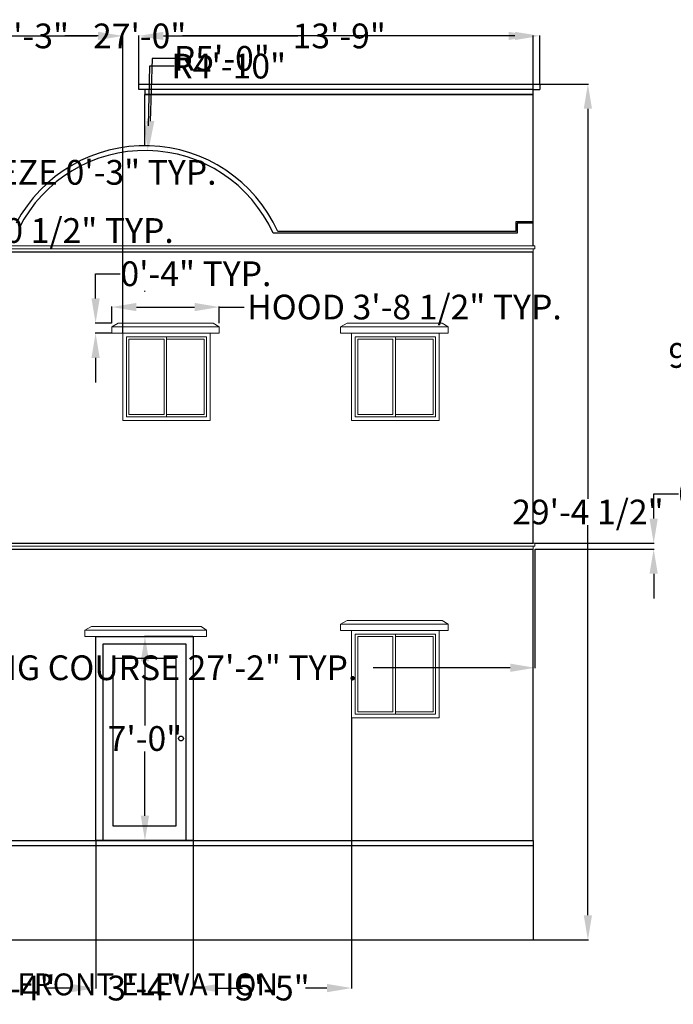
# Model space of a CAD drawing. Units: inches. Extents: x 2393 to 3270, y 740 to 1442.
# Tile 3 of 5: x 2554 to 2823, y 1031 to 1436. Entities that reach past the tile are written whole.
import ezdxf

# ---------------------------------------------------------------- set-up
doc = ezdxf.new("R2010")
doc.units = ezdxf.units.IN
doc.header["$MEASUREMENT"] = 0
for name, color, linetype, lineweight in [('A-ANNO-DIMS', 2, 'Continuous', 18), ('A-ANNO-TITL', 7, 'Continuous', 25), ('A-DOOR', 3, 'Continuous', 25), ('A-ELEV', 7, 'Continuous', 30), ('A-ELEV-TRIM', 8, 'Continuous', 13), ('A-GLAZ', 4, 'Continuous', 18), ('A-ROOF', 7, 'Continuous', 25)]:
    doc.layers.add(name, color=color, linetype=linetype, lineweight=lineweight)
doc.styles.get("Standard").update_dxf_attribs({"font": 'arial.ttf'})
doc.dimstyles.get("Standard").update_dxf_attribs({"dimtxt": 10.18, "dimasz": 10.18, "dimexe": 0.18, "dimexo": 0.0625, "dimgap": 0.09, "dimtad": 0, "dimtih": 1, "dimtoh": 1, "dimdec": 0, "dimzin": 0, "dimdsep": 46, "dimlunit": 3, "dimtxsty": 'Standard', "dimcen": 0.09, "dimadec": 0, "dimazin": 0, "dimtfac": 1, "dimtdec": 0, "dimtofl": 0, "dimtmove": 0, "dimatfit": 3, "dimfxl": 1, "dimtolj": 1, "dimtzin": 0, "dimarcsym": 0})

# ---------------------------------------------------------------- blocks, each defined once
blk = doc.blocks.new('*U7')
blk.add_lwpolyline([(3.12, 0.01), (0.12, 0.01), (0.12, 84.01), (40.12, 84.01), (40.12, 0.01), (37.12, 0.01)])
for points in [[(37.12, 80.99), (37.12, 0.01), (3.12, 0.01), (3.12, 80.99)], [(33.12, 6.01), (33.12, 74.99), (7.12, 74.99), (7.12, 6.01)]]:
    blk.add_lwpolyline(points, close=True)
blk.add_circle((35.12, 42.01), 1)
blk = doc.blocks.new('*U4')
for p, q in [((1.5, 1.5), (1.5, 34.5)), ((1.5, 34.5), (18, 34.5)), ((18, 1.5), (18, 34.5)), ((18, 34.5), (34.5, 34.5)), ((34.5, 34.5), (34.5, 1.5)), ((18, 1.5), (1.5, 1.5)), ((34.5, 1.5), (18, 1.5))]:
    blk.add_line(p, q)
blk.add_lwpolyline([(0, 0), (0, 36), (36, 36), (36, 0)], close=True)
for points in [[(17, 33.5), (17, 2.5), (2.5, 2.5), (2.5, 33.5), (17, 33.5)], [(18, 33.5), (33.5, 33.5), (33.5, 2.5), (18, 2.5)]]:
    blk.add_lwpolyline(points)
blk = doc.blocks.new('WIN-HEAD-HOOD-ELEV')
for p, q in [((0, 2.55), (2.7, 4.11)), ((2.7, 4.11), (41.79, 4.11)), ((41.79, 4.11), (44.29, 2.55)), ((0, 0), (0, 2.55)), ((0, 2.55), (44.29, 2.55)), ((0, 0), (4.55, 0)), ((44.29, 0), (40.55, 0)), ((44.29, 2.55), (44.29, 0))]:
    blk.add_line(p, q)
blk = doc.blocks.new('FACADE-STRING-COURSE')
for p, q in [((0.49, 2.4), (0, 2.4)), ((0, 2.4), (0, 1.23)), ((0, 1.23), (1.17, 1.23)), ((0.49, 2.4), (325.84, 2.4)), ((325.84, 1.23), (325.17, 1.23)), ((325.84, 2.4), (325.84, 1.23))]:
    blk.add_line(p, q)
blk.add_lwpolyline([(1.17, 0), (325.17, 0), (325.17, 1.23), (1.17, 1.23)], close=True)
blk = doc.blocks.new('*D36')
at = {"layer": 'A-ANNO-DIMS', "color": 0, "lineweight": -2, "transparency": 16777216}
for p, q in [((2591.91, 1311.5), (2591.91, 1318.26)), ((2602.09, 1318.08), (2626.02, 1318.08)), ((2636.2, 1311.5), (2636.2, 1318.26)), ((2636.2, 1318.08), (2646.38, 1318.08))]:
    blk.add_line(p, q, dxfattribs=at)
at = {"layer": 'A-ANNO-DIMS', "color": 0, "transparency": 16777216}
for points in [[(2602.09, 1319.77), (2602.09, 1316.38), (2591.91, 1318.08)], [(2626.02, 1319.77), (2626.02, 1316.38), (2636.2, 1318.08)]]:
    blk.add_solid(points, dxfattribs=at)
at = {"layer": 'Defpoints', "color": 0, "transparency": 16777216}
for p in [(2636.2, 1318.08), (2591.91, 1311.43), (2636.2, 1311.43)]:
    blk.add_point(p, dxfattribs=at)
at = {"layer": 'A-ANNO-DIMS', "color": 0, "transparency": 16777216, "insert": (2712.39, 1318.08), "char_height": 10.18, "attachment_point": 5}
blk.add_mtext('\\A1;HOOD 3\'-8 1/2" TYP.', dxfattribs=at)
blk = doc.blocks.new('*D37')
at = {"layer": 'A-ANNO-DIMS', "color": 0, "lineweight": -2, "transparency": 16777216}
for p, q in [((2585.27, 1321.61), (2585.27, 1331.79)), ((2585.27, 1331.79), (2595.45, 1331.79)), ((2591.85, 1311.43), (2585.09, 1311.43)), ((2591.85, 1307.33), (2585.09, 1307.33)), ((2585.27, 1297.15), (2585.27, 1286.97))]:
    blk.add_line(p, q, dxfattribs=at)
at = {"layer": 'A-ANNO-DIMS', "color": 0, "transparency": 16777216}
for points in [[(2583.57, 1321.61), (2586.97, 1321.61), (2585.27, 1311.43)], [(2583.57, 1297.15), (2586.97, 1297.15), (2585.27, 1307.33)]]:
    blk.add_solid(points, dxfattribs=at)
at = {"layer": 'Defpoints', "color": 0, "transparency": 16777216}
for p in [(2585.27, 1311.43), (2591.91, 1311.43), (2591.91, 1307.33)]:
    blk.add_point(p, dxfattribs=at)
at = {"layer": 'A-ANNO-DIMS', "color": 0, "transparency": 16777216, "insert": (2626.57, 1331.79), "char_height": 10.18, "attachment_point": 5}
blk.add_mtext('\\A1;0\'-4" TYP.', dxfattribs=at)
blk = doc.blocks.new('*D38')
at = {"layer": 'A-ANNO-DIMS', "color": 0, "lineweight": -2, "transparency": 16777216}
for p, q in [((2511.53, 1363.37), (2511.53, 1373.55)), ((2511.53, 1373.55), (2521.71, 1373.55)), ((2511.12, 1353.19), (2511.71, 1353.19)), ((2511.12, 1350.06), (2511.71, 1350.06)), ((2511.53, 1339.88), (2511.53, 1329.7))]:
    blk.add_line(p, q, dxfattribs=at)
at = {"layer": 'A-ANNO-DIMS', "color": 0, "transparency": 16777216}
for points in [[(2509.83, 1363.37), (2513.22, 1363.37), (2511.53, 1353.19)], [(2509.83, 1339.88), (2513.22, 1339.88), (2511.53, 1350.06)]]:
    blk.add_solid(points, dxfattribs=at)
at = {"layer": 'Defpoints', "color": 0, "transparency": 16777216}
for p in [(2511.06, 1353.19), (2511.06, 1350.06), (2511.53, 1353.19)]:
    blk.add_point(p, dxfattribs=at)
at = {"layer": 'A-ANNO-DIMS', "color": 0, "transparency": 16777216, "insert": (2579.79, 1373.55), "char_height": 10.18, "attachment_point": 5}
blk.add_mtext('\\A1;FRIEZE 0\'-3" TYP.', dxfattribs=at)
blk = doc.blocks.new('*D39')
at = {"layer": 'A-ANNO-DIMS', "color": 0, "lineweight": -2, "transparency": 16777216}
for p, q in [((2500.38, 1349.6), (2490.2, 1349.6)), ((2510.56, 1350), (2510.56, 1349.42)), ((2511.06, 1350), (2511.06, 1349.42)), ((2521.24, 1349.6), (2531.42, 1349.6))]:
    blk.add_line(p, q, dxfattribs=at)
at = {"layer": 'A-ANNO-DIMS', "color": 0, "transparency": 16777216}
for points in [[(2500.38, 1351.29), (2500.38, 1347.9), (2510.56, 1349.6)], [(2521.24, 1351.29), (2521.24, 1347.9), (2511.06, 1349.6)]]:
    blk.add_solid(points, dxfattribs=at)
at = {"layer": 'Defpoints', "color": 0, "transparency": 16777216}
for p in [(2510.56, 1350.06), (2511.06, 1350.06), (2511.06, 1349.6)]:
    blk.add_point(p, dxfattribs=at)
at = {"layer": 'A-ANNO-DIMS', "color": 0, "transparency": 16777216, "insert": (2574.39, 1349.6), "char_height": 10.18, "attachment_point": 5}
blk.add_mtext('\\A1;0\'-0 1/2" TYP.', dxfattribs=at)
blk = doc.blocks.new('*D40')
at = {"layer": 'A-ANNO-DIMS', "color": 0, "lineweight": -2, "transparency": 16777216}
for p, q in [((2440.26, 1218.37), (2440.26, 1169.38)), ((2766.1, 1218.37), (2766.1, 1169.38)), ((2450.44, 1169.56), (2506.89, 1169.56)), ((2755.92, 1169.56), (2699.46, 1169.56))]:
    blk.add_line(p, q, dxfattribs=at)
at = {"layer": 'A-ANNO-DIMS', "color": 0, "transparency": 16777216}
for points in [[(2450.44, 1171.25), (2450.44, 1167.86), (2440.26, 1169.56)], [(2755.92, 1171.25), (2755.92, 1167.86), (2766.1, 1169.56)]]:
    blk.add_solid(points, dxfattribs=at)
at = {"layer": 'Defpoints', "color": 0, "transparency": 16777216}
for p in [(2440.26, 1218.43), (2766.1, 1218.43), (2766.1, 1169.56)]:
    blk.add_point(p, dxfattribs=at)
at = {"layer": 'A-ANNO-DIMS', "color": 0, "transparency": 16777216, "insert": (2603.18, 1169.56), "char_height": 10.18, "attachment_point": 5}
blk.add_mtext('\\A1;STRING COURSE 27\'-2" TYP.', dxfattribs=at)
blk = doc.blocks.new('*D41')
at = {"layer": 'A-ANNO-DIMS', "color": 0, "lineweight": -2, "transparency": 16777216}
for p, q in [((2814.97, 1231.01), (2814.97, 1241.19)), ((2814.97, 1241.19), (2825.15, 1241.19)), ((2766.16, 1220.83), (2815.15, 1220.83)), ((2766.16, 1218.43), (2815.15, 1218.43)), ((2814.97, 1208.25), (2814.97, 1198.07))]:
    blk.add_line(p, q, dxfattribs=at)
at = {"layer": 'A-ANNO-DIMS', "color": 0, "transparency": 16777216}
for points in [[(2813.27, 1231.01), (2816.67, 1231.01), (2814.97, 1220.83)], [(2813.27, 1208.25), (2816.67, 1208.25), (2814.97, 1218.43)]]:
    blk.add_solid(points, dxfattribs=at)
at = {"layer": 'Defpoints', "color": 0, "transparency": 16777216}
for p in [(2766.1, 1220.83), (2814.97, 1220.83), (2766.1, 1218.43)]:
    blk.add_point(p, dxfattribs=at)
at = {"layer": 'A-ANNO-DIMS', "color": 0, "transparency": 16777216, "insert": (2868.13, 1241.19), "char_height": 10.18, "attachment_point": 5}
blk.add_mtext('\\A1;0\'-2 1/2" TYP.', dxfattribs=at)
blk = doc.blocks.new('*D57')
at = {"layer": 'A-ANNO-DIMS', "color": 0, "lineweight": -2, "transparency": 16777216}
for p, q in [((2441.43, 1353.25), (2441.43, 1429.9)), ((2451.61, 1429.72), (2585.76, 1429.72)), ((2755.25, 1429.72), (2621.09, 1429.72)), ((2765.43, 1353.25), (2765.43, 1429.9))]:
    blk.add_line(p, q, dxfattribs=at)
at = {"layer": 'A-ANNO-DIMS', "color": 0, "transparency": 16777216}
for points in [[(2451.61, 1431.41), (2451.61, 1428.02), (2441.43, 1429.72)], [(2755.25, 1431.41), (2755.25, 1428.02), (2765.43, 1429.72)]]:
    blk.add_solid(points, dxfattribs=at)
at = {"layer": 'Defpoints', "color": 0, "transparency": 16777216}
for p in [(2765.43, 1429.72), (2441.43, 1353.19), (2765.43, 1353.19)]:
    blk.add_point(p, dxfattribs=at)
at = {"layer": 'A-ANNO-DIMS', "color": 0, "transparency": 16777216, "insert": (2603.43, 1429.72), "char_height": 10.18, "attachment_point": 5}
blk.add_mtext('\\A1;27\'-0"', dxfattribs=at)
blk = doc.blocks.new('*D58')
at = {"layer": 'A-ANNO-DIMS', "color": 0, "lineweight": -2, "transparency": 16777216}
for p, q in [((2768.12, 1409.88), (2788.08, 1409.88)), ((2787.9, 1399.7), (2787.9, 1239.05)), ((2787.9, 1067.68), (2787.9, 1228.34)), ((2765.49, 1057.5), (2788.08, 1057.5))]:
    blk.add_line(p, q, dxfattribs=at)
at = {"layer": 'A-ANNO-DIMS', "color": 0, "transparency": 16777216}
for points in [[(2786.2, 1399.7), (2789.59, 1399.7), (2787.9, 1409.88)], [(2786.2, 1067.68), (2789.59, 1067.68), (2787.9, 1057.5)]]:
    blk.add_solid(points, dxfattribs=at)
at = {"layer": 'Defpoints', "color": 0, "transparency": 16777216}
for p in [(2768.06, 1409.88), (2787.9, 1409.88), (2765.43, 1057.5)]:
    blk.add_point(p, dxfattribs=at)
at = {"layer": 'A-ANNO-DIMS', "color": 0, "transparency": 16777216, "insert": (2787.9, 1233.69), "char_height": 10.18, "attachment_point": 5}
blk.add_mtext('\\A1;29\'-4 1/2"', dxfattribs=at)
blk = doc.blocks.new('*D66')
at = {"layer": 'A-ANNO-DIMS', "color": 0, "lineweight": -2, "transparency": 16777216}
for p, q in [((2625.36, 1182.43), (2605.41, 1182.43)), ((2605.59, 1172.25), (2605.59, 1145.72)), ((2605.59, 1108.61), (2605.59, 1135.14)), ((2625.36, 1098.43), (2605.41, 1098.43))]:
    blk.add_line(p, q, dxfattribs=at)
at = {"layer": 'A-ANNO-DIMS', "color": 0, "transparency": 16777216}
for points in [[(2603.89, 1172.25), (2607.29, 1172.25), (2605.59, 1182.43)], [(2603.89, 1108.61), (2607.29, 1108.61), (2605.59, 1098.43)]]:
    blk.add_solid(points, dxfattribs=at)
at = {"layer": 'Defpoints', "color": 0, "transparency": 16777216}
for p in [(2605.59, 1182.43), (2625.43, 1182.43), (2625.43, 1098.43)]:
    blk.add_point(p, dxfattribs=at)
at = {"layer": 'A-ANNO-DIMS', "color": 0, "transparency": 16777216, "insert": (2605.59, 1140.43), "char_height": 10.18, "attachment_point": 5}
blk.add_mtext('\\A1;7\'-0"', dxfattribs=at)
blk = doc.blocks.new('*D69')
at = {"layer": 'A-ANNO-DIMS', "color": 0, "lineweight": -2, "transparency": 16777216}
for p, q in [((2521.51, 1148.87), (2521.51, 1037.49)), ((2585.43, 1098.37), (2585.43, 1037.49)), ((2531.69, 1037.67), (2539.85, 1037.67)), ((2575.25, 1037.67), (2567.09, 1037.67))]:
    blk.add_line(p, q, dxfattribs=at)
at = {"layer": 'A-ANNO-DIMS', "color": 0, "transparency": 16777216}
for points in [[(2531.69, 1039.37), (2531.69, 1035.97), (2521.51, 1037.67)], [(2575.25, 1039.37), (2575.25, 1035.97), (2585.43, 1037.67)]]:
    blk.add_solid(points, dxfattribs=at)
at = {"layer": 'Defpoints', "color": 0, "transparency": 16777216}
for p in [(2521.51, 1148.93), (2585.43, 1098.43), (2585.43, 1037.67)]:
    blk.add_point(p, dxfattribs=at)
at = {"layer": 'A-ANNO-DIMS', "color": 0, "transparency": 16777216, "insert": (2553.47, 1037.67), "char_height": 10.18, "attachment_point": 5}
blk.add_mtext('\\A1;5\'-4"', dxfattribs=at)
blk = doc.blocks.new('*D70')
at = {"layer": 'A-ANNO-DIMS', "color": 0, "lineweight": -2, "transparency": 16777216}
for p, q in [((2585.43, 1098.37), (2585.43, 1037.49)), ((2625.43, 1098.37), (2625.43, 1037.49)), ((2575.25, 1037.67), (2565.07, 1037.67)), ((2635.61, 1037.67), (2645.79, 1037.67))]:
    blk.add_line(p, q, dxfattribs=at)
at = {"layer": 'A-ANNO-DIMS', "color": 0, "transparency": 16777216}
for points in [[(2575.25, 1039.37), (2575.25, 1035.97), (2585.43, 1037.67)], [(2635.61, 1039.37), (2635.61, 1035.97), (2625.43, 1037.67)]]:
    blk.add_solid(points, dxfattribs=at)
at = {"layer": 'Defpoints', "color": 0, "transparency": 16777216}
for p in [(2585.43, 1098.43), (2625.43, 1098.43), (2625.43, 1037.67)]:
    blk.add_point(p, dxfattribs=at)
at = {"layer": 'A-ANNO-DIMS', "color": 0, "transparency": 16777216, "insert": (2605.43, 1037.67), "char_height": 10.18, "attachment_point": 5}
blk.add_mtext('\\A1;3\'-4"', dxfattribs=at)
blk = doc.blocks.new('*D71')
at = {"layer": 'A-ANNO-DIMS', "color": 0, "lineweight": -2, "transparency": 16777216}
for p, q in [((2690.67, 1148.87), (2690.67, 1037.49)), ((2625.43, 1098.37), (2625.43, 1037.49)), ((2635.61, 1037.67), (2644.43, 1037.67)), ((2680.49, 1037.67), (2671.67, 1037.67))]:
    blk.add_line(p, q, dxfattribs=at)
at = {"layer": 'A-ANNO-DIMS', "color": 0, "transparency": 16777216}
for points in [[(2635.61, 1039.37), (2635.61, 1035.97), (2625.43, 1037.67)], [(2680.49, 1039.37), (2680.49, 1035.97), (2690.67, 1037.67)]]:
    blk.add_solid(points, dxfattribs=at)
at = {"layer": 'Defpoints', "color": 0, "transparency": 16777216}
for p in [(2690.67, 1148.93), (2625.43, 1098.43), (2690.67, 1037.67)]:
    blk.add_point(p, dxfattribs=at)
at = {"layer": 'A-ANNO-DIMS', "color": 0, "transparency": 16777216, "insert": (2658.05, 1037.67), "char_height": 10.18, "attachment_point": 5}
blk.add_mtext('\\A1;5\'-5"', dxfattribs=at)
blk = doc.blocks.new('*D72')
at = {"layer": 'A-ANNO-DIMS', "color": 0, "lineweight": -2, "transparency": 16777216}
for p, q in [((2521.51, 1307.39), (2521.51, 1429.9)), ((2531.69, 1429.72), (2545.34, 1429.72)), ((2586.29, 1429.72), (2572.64, 1429.72)), ((2596.47, 1307.39), (2596.47, 1429.9))]:
    blk.add_line(p, q, dxfattribs=at)
at = {"layer": 'A-ANNO-DIMS', "color": 0, "transparency": 16777216}
for points in [[(2531.69, 1431.41), (2531.69, 1428.02), (2521.51, 1429.72)], [(2586.29, 1431.41), (2586.29, 1428.02), (2596.47, 1429.72)]]:
    blk.add_solid(points, dxfattribs=at)
at = {"layer": 'Defpoints', "color": 0, "transparency": 16777216}
for p in [(2596.47, 1429.72), (2521.51, 1307.33), (2596.47, 1307.33)]:
    blk.add_point(p, dxfattribs=at)
at = {"layer": 'A-ANNO-DIMS', "color": 0, "transparency": 16777216, "insert": (2558.99, 1429.72), "char_height": 10.18, "attachment_point": 5}
blk.add_mtext('\\A1;6\'-3"', dxfattribs=at)
blk = doc.blocks.new('*D73')
at = {"layer": 'A-ANNO-DIMS', "color": 0, "lineweight": -2, "transparency": 16777216}
for p, q in [((2603.04, 1409.94), (2603.04, 1429.9)), ((2613.22, 1429.72), (2668.46, 1429.72)), ((2757.88, 1429.72), (2702.65, 1429.72)), ((2768.06, 1409.94), (2768.06, 1429.9))]:
    blk.add_line(p, q, dxfattribs=at)
at = {"layer": 'A-ANNO-DIMS', "color": 0, "transparency": 16777216}
for points in [[(2613.22, 1431.41), (2613.22, 1428.02), (2603.04, 1429.72)], [(2757.88, 1431.41), (2757.88, 1428.02), (2768.06, 1429.72)]]:
    blk.add_solid(points, dxfattribs=at)
at = {"layer": 'Defpoints', "color": 0, "transparency": 16777216}
for p in [(2768.06, 1429.72), (2603.04, 1409.88), (2768.06, 1409.88)]:
    blk.add_point(p, dxfattribs=at)
at = {"layer": 'A-ANNO-DIMS', "color": 0, "transparency": 16777216, "insert": (2685.55, 1429.72), "char_height": 10.18, "attachment_point": 5}
blk.add_mtext('\\A1;13\'-9"', dxfattribs=at)
blk = doc.blocks.new('*D79')
at = {"layer": 'A-ANNO-DIMS', "color": 0, "lineweight": -2, "transparency": 16777216}
for p, q in [((2869.02, 1357.55), (2840.03, 1357.55)), ((2840.21, 1347.37), (2840.21, 1303.44)), ((2840.21, 1248.94), (2840.21, 1292.87)), ((2869.02, 1238.76), (2840.03, 1238.76))]:
    blk.add_line(p, q, dxfattribs=at)
at = {"layer": 'A-ANNO-DIMS', "color": 0, "transparency": 16777216}
for points in [[(2838.51, 1347.37), (2841.91, 1347.37), (2840.21, 1357.55)], [(2838.51, 1248.94), (2841.91, 1248.94), (2840.21, 1238.76)]]:
    blk.add_solid(points, dxfattribs=at)
at = {"layer": 'Defpoints', "color": 0, "transparency": 16777216}
for p in [(2840.21, 1357.55), (2869.08, 1357.55), (2869.08, 1238.76)]:
    blk.add_point(p, dxfattribs=at)
at = {"layer": 'A-ANNO-DIMS', "color": 0, "transparency": 16777216, "insert": (2840.21, 1298.16), "char_height": 10.18, "attachment_point": 5}
blk.add_mtext('\\A1;9\'-11"', dxfattribs=at)
blk = doc.blocks.new('*D84')
at = {"layer": 'A-ANNO-DIMS', "color": 0, "lineweight": -2, "transparency": 16777216}
for p, q in [((2608.56, 1420.45), (2607.76, 1394.68)), ((2618.74, 1420.45), (2608.56, 1420.45)), ((2605.49, 1324.61), (2605.67, 1324.61)), ((2605.58, 1324.52), (2605.58, 1324.7))]:
    blk.add_line(p, q, dxfattribs=at)
at = {"layer": 'A-ANNO-DIMS', "color": 0, "transparency": 16777216}
blk.add_solid([(2606.06, 1394.74), (2609.45, 1394.63), (2607.44, 1384.51)], dxfattribs=at)
at = {"layer": 'Defpoints', "color": 0, "transparency": 16777216}
for p in [(2607.44, 1384.51), (2605.58, 1324.61)]:
    blk.add_point(p, dxfattribs=at)
at = {"layer": 'A-ANNO-DIMS', "color": 0, "transparency": 16777216, "insert": (2637.23, 1420.45), "char_height": 10.18, "attachment_point": 5}
blk.add_mtext('\\A1;R5\'-0"', dxfattribs=at)
blk = doc.blocks.new('*D85')
at = {"layer": 'A-ANNO-DIMS', "color": 0, "lineweight": -2, "transparency": 16777216}
for p, q in [((2607.45, 1417.28), (2606.95, 1392.7)), ((2617.63, 1417.28), (2607.45, 1417.28)), ((2605.49, 1324.61), (2605.67, 1324.61)), ((2605.58, 1324.52), (2605.58, 1324.7))]:
    blk.add_line(p, q, dxfattribs=at)
at = {"layer": 'A-ANNO-DIMS', "color": 0, "transparency": 16777216}
blk.add_solid([(2605.26, 1392.74), (2608.65, 1392.67), (2606.75, 1382.53)], dxfattribs=at)
at = {"layer": 'Defpoints', "color": 0, "transparency": 16777216}
for p in [(2606.75, 1382.53), (2605.58, 1324.61)]:
    blk.add_point(p, dxfattribs=at)
at = {"layer": 'A-ANNO-DIMS', "color": 0, "transparency": 16777216, "insert": (2640.07, 1417.28), "char_height": 10.18, "attachment_point": 5}
blk.add_mtext('\\A1;R4\'-10"', dxfattribs=at)

msp = doc.modelspace()

# ---------------------------------------------------------------- linework, layer by layer
at = {"layer": 'A-ELEV'}
for p, q in [((2441.43, 1340.83), (2765.43, 1340.83)), ((2765.43, 1220.83), (2765.43, 1340.83)), ((2441.43, 1220.83), (2765.43, 1220.83)), ((2441.43, 1218.43), (2765.43, 1218.43)), ((2765.43, 1098.43), (2765.43, 1218.43)), ((2441.43, 1098.43), (2765.43, 1098.43)), ((2441.43, 1096.43), (2765.43, 1096.43)), ((2765.43, 1098.43), (2765.43, 1057.5)), ((2441.43, 1057.5), (2765.43, 1057.5))]:
    msp.add_line(p, q, dxfattribs=at)
at = {"layer": 'A-ELEV-TRIM'}
for p, q in [((2580.87, 1184.98), (2583.57, 1186.54)), ((2580.87, 1182.43), (2580.87, 1184.98)), ((2580.87, 1184.98), (2628.62, 1184.98)), ((2583.57, 1186.54), (2628.67, 1186.54)), ((2628.62, 1184.98), (2630.87, 1184.98)), ((2630.87, 1184.98), (2628.67, 1186.54)), ((2630.87, 1184.98), (2630.87, 1182.43)), ((2630.87, 1184.98), (2630.87, 1184.98)), ((2580.87, 1182.43), (2585.43, 1182.43)), ((2628.62, 1182.43), (2625.43, 1182.43)), ((2630.87, 1182.43), (2628.62, 1182.43))]:
    msp.add_line(p, q, dxfattribs=at)
at = {"layer": 'A-ROOF'}
for p, q in [((2603.04, 1407.63), (2603.04, 1409.88)), ((2603.04, 1409.88), (2768.06, 1409.88)), ((2605.58, 1407.63), (2603.04, 1407.63)), ((2765.43, 1407.63), (2768.06, 1407.63)), ((2768.06, 1409.88), (2768.06, 1407.63)), ((2605.58, 1384.54), (2605.58, 1405.54)), ((2605.58, 1405.54), (2765.43, 1405.54)), ((2765.43, 1353.19), (2765.43, 1405.54)), ((2765.43, 1353.19), (2758.26, 1353.19)), ((2758.26, 1353.19), (2758.26, 1349.23)), ((2765.43, 1352.66), (2758.81, 1352.66)), ((2758.81, 1352.66), (2758.81, 1348.45)), ((2765.43, 1343.22), (2765.43, 1353.19)), ((2758.81, 1348.45), (2658.38, 1348.45)), ((2758.26, 1349.23), (2660.22, 1349.23))]:
    msp.add_line(p, q, dxfattribs=at)
for points in [[(2605.58, 1405.54), (2765.43, 1405.54), (2765.43, 1407.63), (2605.58, 1407.63)], [(2605.58, 1405.54), (2765.43, 1405.54), (2765.43, 1405.54), (2605.58, 1405.54)]]:
    msp.add_lwpolyline(points, close=True, dxfattribs=at)
for radius, start, end in [(59.93, 24.2594, 152.1815), (57.93, 24.2995, 153.3937)]:
    msp.add_arc((2605.58, 1324.61), radius, start, end, dxfattribs=at)

# ---------------------------------------------------------------- block references
at = {"layer": 'A-DOOR'}
msp.add_blockref('*U7', (2585.3, 1098.42), dxfattribs=at)
at = {"layer": 'A-ELEV-TRIM'}
for name, p in [('FACADE-STRING-COURSE', (2440.26, 1340.83)), ('WIN-HEAD-HOOD-ELEV', (2591.91, 1307.33)), ('WIN-HEAD-HOOD-ELEV', (2686.11, 1307.33)), ('FACADE-STRING-COURSE', (2440.26, 1218.43)), ('WIN-HEAD-HOOD-ELEV', (2686.11, 1184.93))]:
    msp.add_blockref(name, p, dxfattribs=at)
at = {"layer": 'A-GLAZ'}
for p in [(2596.47, 1271.33), (2690.67, 1271.33), (2690.67, 1148.93)]:
    msp.add_blockref('*U4', p, dxfattribs=at)

# ---------------------------------------------------------------- texts
at = {"layer": 'A-ANNO-TITL', "insert": (2553.06, 1043.69), "char_height": 9, "attachment_point": 1}
msp.add_mtext_dynamic_manual_height_columns('FRONT ELEVATION', width=140.3126, gutter_width=1, heights=[0], dxfattribs=at)

# ---------------------------------------------------------------- dimensions: what is measured, and where the dimension line sits
at = {"layer": 'A-ANNO-DIMS'}
for base, p1, p2, picture, middle in [((2765.43, 1429.72), (2441.43, 1353.19), (2765.43, 1353.19), '*D57', (2603.43, 1429.72)), ((2596.47, 1429.72), (2521.51, 1307.33), (2596.47, 1307.33), '*D72', (2558.99, 1429.72)), ((2768.06, 1429.72), (2603.04, 1409.88), (2768.06, 1409.88), '*D73', (2685.55, 1429.72)), ((2585.43, 1037.67), (2521.51, 1148.93), (2585.43, 1098.43), '*D69', (2553.47, 1037.67)), ((2690.67, 1037.67), (2625.43, 1098.43), (2690.67, 1148.93), '*D71', (2658.05, 1037.67)), ((2625.43, 1037.67), (2585.43, 1098.43), (2625.43, 1098.43), '*D70', (2605.43, 1037.67))]:
    dim = msp.add_linear_dim(base=base, p1=p1, p2=p2, dimstyle='Standard', override={"dimdec": 1, "dimlfac": 1, "dimrnd": 0, "dimzin": 1, "dimdsep": 46, "dimlunit": 4, "dimfrac": 2}, dxfattribs=at)
    dim.commit()
    dim.dimension.update_dxf_attribs({"geometry": picture, "text_midpoint": middle})
for mpoint, picture, middle in [((2607.44, 1384.51), '*D84', (2637.23, 1420.45)), ((2606.75, 1382.53), '*D85', (2640.07, 1417.28))]:
    dim = msp.add_radius_dim(center=(2605.58, 1324.61), mpoint=mpoint, dimstyle='Standard', override={"dimdec": 1, "dimlfac": 1, "dimrnd": 0, "dimzin": 1, "dimdsep": 46, "dimlunit": 4, "dimfrac": 2}, dxfattribs=at)
    dim.commit()
    dim.dimension.update_dxf_attribs({"geometry": picture, "text_midpoint": middle, "dimtype": 164})
for base, p1, p2, picture, middle in [((2787.9, 1409.88), (2765.43, 1057.5), (2768.06, 1409.88), '*D58', (2787.9, 1233.69)), ((2840.21, 1357.55), (2869.08, 1238.76), (2869.08, 1357.55), '*D79', (2840.21, 1298.16)), ((2605.59, 1182.43), (2625.43, 1098.43), (2625.43, 1182.43), '*D66', (2605.59, 1140.43))]:
    dim = msp.add_linear_dim(base=base, p1=p1, p2=p2, angle=90, dimstyle='Standard', override={"dimdec": 1, "dimlfac": 1, "dimrnd": 0, "dimzin": 1, "dimdsep": 46, "dimlunit": 4, "dimfrac": 2}, dxfattribs=at)
    dim.commit()
    dim.dimension.update_dxf_attribs({"geometry": picture, "text_midpoint": middle})
for base, p1, p2, text, picture, middle in [((2511.53, 1353.19), (2511.06, 1350.06), (2511.06, 1353.19), 'FRIEZE <> TYP.', '*D38', (2579.79, 1373.55)), ((2585.27, 1311.43), (2591.91, 1307.33), (2591.91, 1311.43), '<> TYP.', '*D37', (2626.57, 1331.79)), ((2814.97, 1220.83), (2766.1, 1218.43), (2766.1, 1220.83), '<> TYP.', '*D41', (2868.13, 1241.19))]:
    dim = msp.add_linear_dim(base=base, p1=p1, p2=p2, angle=90, text=text, dimstyle='Standard', override={"dimdec": 1, "dimlfac": 1, "dimrnd": 0, "dimzin": 1, "dimdsep": 46, "dimlunit": 4, "dimfrac": 2}, dxfattribs=at)
    dim.commit()
    dim.dimension.update_dxf_attribs({"geometry": picture, "text_midpoint": middle})
for base, p1, p2, text, picture, middle in [((2511.06, 1349.6), (2510.56, 1350.06), (2511.06, 1350.06), '<> TYP.', '*D39', (2574.39, 1349.6)), ((2636.2, 1318.08), (2591.91, 1311.43), (2636.2, 1311.43), 'HOOD <> TYP.', '*D36', (2712.39, 1318.08)), ((2766.1, 1169.56), (2440.26, 1218.43), (2766.1, 1218.43), 'STRING COURSE <> TYP.', '*D40', (2603.18, 1169.56))]:
    dim = msp.add_linear_dim(base=base, p1=p1, p2=p2, text=text, dimstyle='Standard', override={"dimdec": 1, "dimlfac": 1, "dimrnd": 0, "dimzin": 1, "dimdsep": 46, "dimlunit": 4, "dimfrac": 2}, dxfattribs=at)
    dim.commit()
    dim.dimension.update_dxf_attribs({"geometry": picture, "text_midpoint": middle})

doc.saveas('drawing.dxf')
